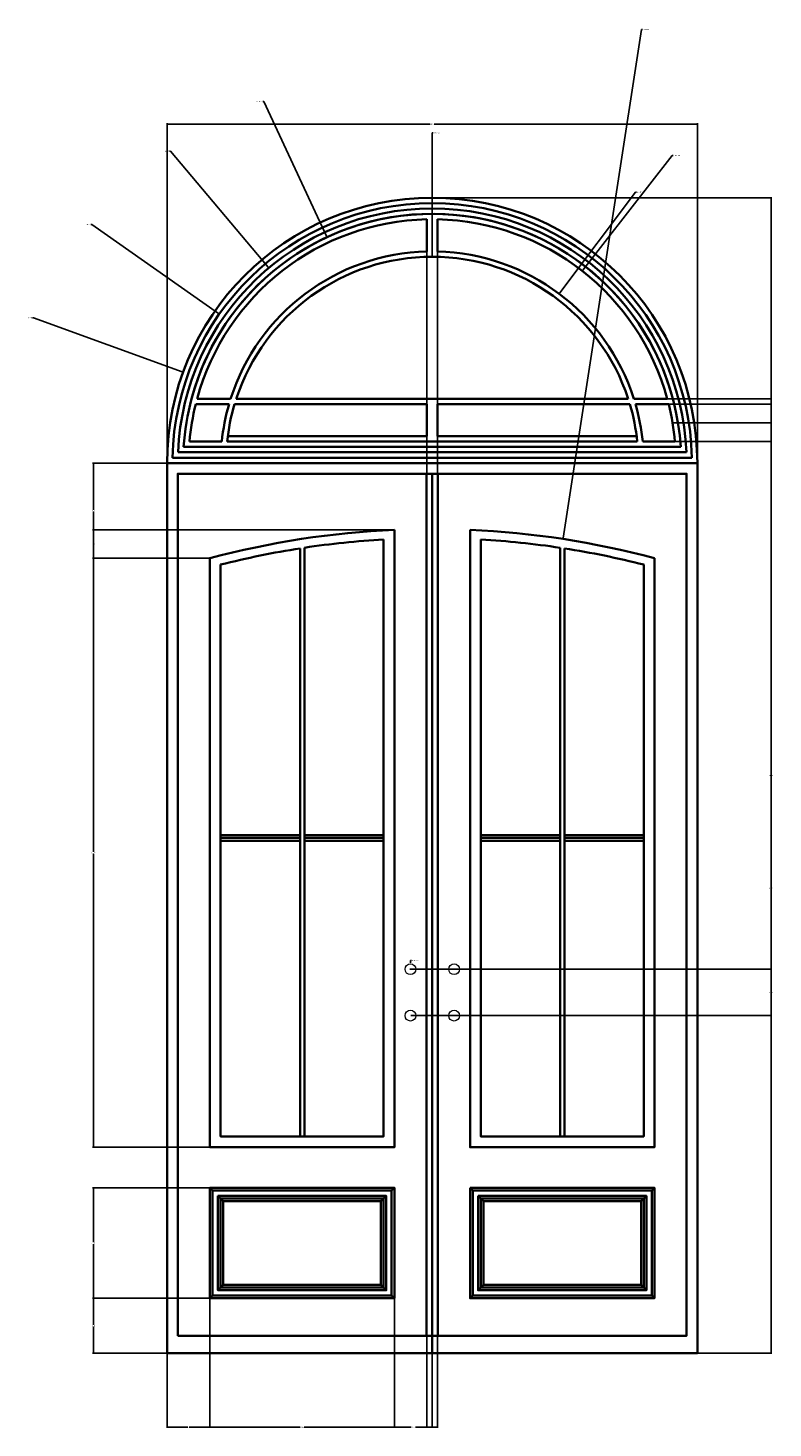
# Model space of a CAD drawing. Units: inches. Extents: x 1318 to 1980, y 617 to 1423.
# Tile 3 of 7: x 1332 to 1471, y 944 to 1205. Entities that reach past the tile are written whole.
import ezdxf

# ---------------------------------------------------------------- set-up
doc = ezdxf.new("R2010")
doc.units = ezdxf.units.IN
doc.header["$MEASUREMENT"] = 0
for name, color, linetype, lineweight in [('A-ANNO-DIMS', 2, 'Continuous', 18), ('A-DOOR', 4, 'Continuous', 35), ('A-DOOR-HDWR', 3, 'Continuous', 18)]:
    doc.layers.add(name, color=color, linetype=linetype, lineweight=lineweight)
doc.styles.get("Standard").update_dxf_attribs({"font": 'arial.ttf'})
doc.dimstyles.get("Standard").update_dxf_attribs({"dimtxt": 0.18, "dimasz": 0.18, "dimexe": 0.18, "dimexo": 0.0625, "dimgap": 0.09, "dimtad": 0, "dimtih": 1, "dimtoh": 1, "dimdec": 0, "dimzin": 0, "dimdsep": 46, "dimlunit": 3, "dimtxsty": 'Standard', "dimcen": 0.09, "dimadec": 0, "dimazin": 0, "dimtfac": 1, "dimtdec": 0, "dimtofl": 0, "dimtmove": 0, "dimatfit": 3, "dimfxl": 1, "dimtolj": 1, "dimtzin": 0, "dimarcsym": 0})

# ---------------------------------------------------------------- blocks, each defined once
blk = doc.blocks.new('DOOR-KNOB-SET')
for centre in [(1.01, 9.67), (9.16, 9.67), (1.01, 1.01), (9.16, 1.01)]:
    blk.add_circle(centre, 1.01)
blk = doc.blocks.new('*D32')
at = {"layer": 'A-ANNO-DIMS', "color": 0, "lineweight": -2, "transparency": 16777216}
for p, q in [((1403.05, 1020.69), (1470.47, 1020.69)), ((1470.29, 1020.51), (1470.29, 989.38)), ((1470.29, 957.88), (1470.29, 989.01)), ((1407.11, 957.7), (1470.47, 957.7))]:
    blk.add_line(p, q, dxfattribs=at)
at = {"layer": 'A-ANNO-DIMS', "color": 0, "transparency": 16777216}
for points in [[(1470.26, 1020.51), (1470.32, 1020.51), (1470.29, 1020.69)], [(1470.26, 957.88), (1470.32, 957.88), (1470.29, 957.7)]]:
    blk.add_solid(points, dxfattribs=at)
at = {"layer": 'Defpoints', "color": 0, "transparency": 16777216}
for p in [(1402.99, 1020.69), (1470.29, 1020.69), (1407.05, 957.7)]:
    blk.add_point(p, dxfattribs=at)
at = {"layer": 'A-ANNO-DIMS', "color": 0, "transparency": 16777216, "insert": (1470.29, 989.2), "char_height": 0.18, "attachment_point": 5}
blk.add_mtext('\\A1;63', dxfattribs=at)
blk = doc.blocks.new('*D33')
at = {"layer": 'A-ANNO-DIMS', "color": 0, "lineweight": -2, "transparency": 16777216}
for p, q in [((1403.05, 1029.36), (1470.47, 1029.36)), ((1470.29, 1029.18), (1470.29, 1025.21)), ((1470.29, 1020.87), (1470.29, 1024.84)), ((1403.05, 1020.69), (1470.47, 1020.69))]:
    blk.add_line(p, q, dxfattribs=at)
at = {"layer": 'A-ANNO-DIMS', "color": 0, "transparency": 16777216}
for points in [[(1470.26, 1029.18), (1470.32, 1029.18), (1470.29, 1029.36)], [(1470.26, 1020.87), (1470.32, 1020.87), (1470.29, 1020.69)]]:
    blk.add_solid(points, dxfattribs=at)
at = {"layer": 'Defpoints', "color": 0, "transparency": 16777216}
for p in [(1402.99, 1029.36), (1470.29, 1029.36), (1402.99, 1020.69)]:
    blk.add_point(p, dxfattribs=at)
at = {"layer": 'A-ANNO-DIMS', "color": 0, "transparency": 16777216, "insert": (1470.29, 1025.03), "char_height": 0.18, "attachment_point": 5}
blk.add_mtext('\\A1;8.663', dxfattribs=at)
blk = doc.blocks.new('*D34')
at = {"layer": 'A-ANNO-DIMS', "color": 0, "lineweight": -2, "transparency": 16777216}
for p, q in [((1357.56, 1123.84), (1357.56, 1187.2)), ((1357.74, 1187.02), (1406.65, 1187.02)), ((1456.36, 1187.02), (1407.44, 1187.02)), ((1456.54, 1123.84), (1456.54, 1187.2))]:
    blk.add_line(p, q, dxfattribs=at)
at = {"layer": 'A-ANNO-DIMS', "color": 0, "transparency": 16777216}
for points in [[(1357.74, 1187.05), (1357.74, 1186.99), (1357.56, 1187.02)], [(1456.36, 1187.05), (1456.36, 1186.99), (1456.54, 1187.02)]]:
    blk.add_solid(points, dxfattribs=at)
at = {"layer": 'Defpoints', "color": 0, "transparency": 16777216}
for p in [(1456.54, 1187.02), (1357.56, 1123.78), (1456.54, 1123.78)]:
    blk.add_point(p, dxfattribs=at)
at = {"layer": 'A-ANNO-DIMS', "color": 0, "transparency": 16777216, "insert": (1407.05, 1187.02), "char_height": 0.18, "attachment_point": 5}
blk.add_mtext('\\A1;98.98', dxfattribs=at)
blk = doc.blocks.new('*D35')
at = {"layer": 'A-ANNO-DIMS', "color": 0, "lineweight": -2, "transparency": 16777216}
for p, q in [((1451.97, 1131.3), (1470.47, 1131.3)), ((1470.29, 1131.12), (1470.29, 1044.68)), ((1470.29, 957.88), (1470.29, 1044.32)), ((1456.6, 957.7), (1470.47, 957.7))]:
    blk.add_line(p, q, dxfattribs=at)
at = {"layer": 'A-ANNO-DIMS', "color": 0, "transparency": 16777216}
for points in [[(1470.26, 1131.12), (1470.32, 1131.12), (1470.29, 1131.3)], [(1470.26, 957.88), (1470.32, 957.88), (1470.29, 957.7)]]:
    blk.add_solid(points, dxfattribs=at)
at = {"layer": 'Defpoints', "color": 0, "transparency": 16777216}
for p in [(1451.91, 1131.3), (1470.29, 1131.3), (1456.54, 957.7)]:
    blk.add_point(p, dxfattribs=at)
at = {"layer": 'A-ANNO-DIMS', "color": 0, "transparency": 16777216, "insert": (1470.29, 1044.5), "char_height": 0.18, "attachment_point": 5}
blk.add_mtext('\\A1;173.6', dxfattribs=at)
blk = doc.blocks.new('*D36')
at = {"layer": 'A-ANNO-DIMS', "color": 0, "lineweight": -2, "transparency": 16777216}
for p, q in [((1407.11, 1173.27), (1470.47, 1173.27)), ((1470.29, 1173.09), (1470.29, 1065.67)), ((1470.29, 957.88), (1470.29, 1065.3)), ((1357.62, 957.7), (1470.47, 957.7))]:
    blk.add_line(p, q, dxfattribs=at)
at = {"layer": 'A-ANNO-DIMS', "color": 0, "transparency": 16777216}
for points in [[(1470.26, 1173.09), (1470.32, 1173.09), (1470.29, 1173.27)], [(1470.26, 957.88), (1470.32, 957.88), (1470.29, 957.7)]]:
    blk.add_solid(points, dxfattribs=at)
at = {"layer": 'Defpoints', "color": 0, "transparency": 16777216}
for p in [(1407.05, 1173.27), (1470.29, 1173.27), (1357.56, 957.7)]:
    blk.add_point(p, dxfattribs=at)
at = {"layer": 'A-ANNO-DIMS', "color": 0, "transparency": 16777216, "insert": (1470.29, 1065.48), "char_height": 0.18, "attachment_point": 5}
blk.add_mtext('\\A1;215.57', dxfattribs=at)
blk = doc.blocks.new('*D37')
at = {"layer": 'A-ANNO-DIMS', "color": 0, "lineweight": -2, "transparency": 16777216}
for p, q in [((1451.249026, 1134.780871), (1470.466544, 1134.780871)), ((1470.286544, 1134.600871), (1470.286544, 1131.460871)), ((1470.286544, 1127.960871), (1470.286544, 1131.100871)), ((1452.422837, 1127.780871), (1470.466544, 1127.780871))]:
    blk.add_line(p, q, dxfattribs=at)
at = {"layer": 'A-ANNO-DIMS', "color": 0, "transparency": 16777216}
for points in [[(1470.256544, 1134.600871), (1470.316544, 1134.600871), (1470.286544, 1134.780871)], [(1470.256544, 1127.960871), (1470.316544, 1127.960871), (1470.286544, 1127.780871)]]:
    blk.add_solid(points, dxfattribs=at)
at = {"layer": 'Defpoints', "color": 0, "transparency": 16777216}
for p in [(1451.186526, 1134.780871), (1470.286544, 1134.780871), (1452.360337, 1127.780871)]:
    blk.add_point(p, dxfattribs=at)
at = {"layer": 'A-ANNO-DIMS', "color": 0, "transparency": 16777216, "insert": (1470.286544, 1131.280871), "char_height": 0.18, "attachment_point": 5}
blk.add_mtext('\\A1;7', dxfattribs=at)
blk = doc.blocks.new('*D38')
at = {"layer": 'A-ANNO-DIMS', "color": 0, "lineweight": -2, "transparency": 16777216}
for p, q in [((1450.99, 1135.78), (1470.47, 1135.78)), ((1451.25, 1134.78), (1470.47, 1134.78)), ((1470.29, 1135.6), (1470.29, 1135.46)), ((1470.29, 1134.96), (1470.29, 1135.1))]:
    blk.add_line(p, q, dxfattribs=at)
at = {"layer": 'A-ANNO-DIMS', "color": 0, "transparency": 16777216}
for points in [[(1470.26, 1135.6), (1470.32, 1135.6), (1470.29, 1135.78)], [(1470.26, 1134.96), (1470.32, 1134.96), (1470.29, 1134.78)]]:
    blk.add_solid(points, dxfattribs=at)
at = {"layer": 'Defpoints', "color": 0, "transparency": 16777216}
for p in [(1450.93, 1135.78), (1451.19, 1134.78), (1470.29, 1135.78)]:
    blk.add_point(p, dxfattribs=at)
at = {"layer": 'A-ANNO-DIMS', "color": 0, "transparency": 16777216, "insert": (1470.29, 1135.28), "char_height": 0.18, "attachment_point": 5}
blk.add_mtext('\\A1;1', dxfattribs=at)
blk = doc.blocks.new('*D39')
at = {"layer": 'A-ANNO-DIMS', "color": 0, "lineweight": -2, "transparency": 16777216}
for p, q in [((1406.05, 1163.19), (1406.05, 943.77)), ((1408.05, 1163.19), (1408.05, 943.77)), ((1406.23, 943.95), (1406.9, 943.95)), ((1407.87, 943.95), (1407.2, 943.95))]:
    blk.add_line(p, q, dxfattribs=at)
at = {"layer": 'A-ANNO-DIMS', "color": 0, "transparency": 16777216}
for points in [[(1406.23, 943.98), (1406.23, 943.92), (1406.05, 943.95)], [(1407.87, 943.98), (1407.87, 943.92), (1408.05, 943.95)]]:
    blk.add_solid(points, dxfattribs=at)
at = {"layer": 'Defpoints', "color": 0, "transparency": 16777216}
for p in [(1406.05, 1163.26), (1408.05, 1163.26), (1408.05, 943.95)]:
    blk.add_point(p, dxfattribs=at)
at = {"layer": 'A-ANNO-DIMS', "color": 0, "transparency": 16777216, "insert": (1407.05, 943.95), "char_height": 0.18, "attachment_point": 5}
blk.add_mtext('\\A1;2', dxfattribs=at)
blk = doc.blocks.new('*D40')
at = {"layer": 'A-ANNO-DIMS', "color": 0, "lineweight": -2, "transparency": 16777216}
for p, q in [((1399.92, 1111.33), (1343.63, 1111.33)), ((1343.81, 1111.15), (1343.81, 1108.86)), ((1343.81, 1106.2), (1343.81, 1108.49)), ((1365.5, 1106.02), (1343.63, 1106.02))]:
    blk.add_line(p, q, dxfattribs=at)
at = {"layer": 'A-ANNO-DIMS', "color": 0, "transparency": 16777216}
for points in [[(1343.78, 1111.15), (1343.84, 1111.15), (1343.81, 1111.33)], [(1343.78, 1106.2), (1343.84, 1106.2), (1343.81, 1106.02)]]:
    blk.add_solid(points, dxfattribs=at)
at = {"layer": 'Defpoints', "color": 0, "transparency": 16777216}
for p in [(1343.81, 1111.33), (1399.98, 1111.33), (1365.56, 1106.02)]:
    blk.add_point(p, dxfattribs=at)
at = {"layer": 'A-ANNO-DIMS', "color": 0, "transparency": 16777216, "insert": (1343.81, 1108.68), "char_height": 0.18, "attachment_point": 5}
blk.add_mtext('\\A1;5.306', dxfattribs=at)
blk = doc.blocks.new('*D41')
at = {"layer": 'A-ANNO-DIMS', "color": 0, "lineweight": -2, "transparency": 16777216}
for p, q in [((1365.56, 967.92), (1365.56, 943.77)), ((1357.56, 957.63), (1357.56, 943.77)), ((1357.74, 943.95), (1361.41, 943.95)), ((1365.38, 943.95), (1361.71, 943.95))]:
    blk.add_line(p, q, dxfattribs=at)
at = {"layer": 'A-ANNO-DIMS', "color": 0, "transparency": 16777216}
for points in [[(1357.74, 943.98), (1357.74, 943.92), (1357.56, 943.95)], [(1365.38, 943.98), (1365.38, 943.92), (1365.56, 943.95)]]:
    blk.add_solid(points, dxfattribs=at)
at = {"layer": 'Defpoints', "color": 0, "transparency": 16777216}
for p in [(1365.56, 967.98), (1357.56, 957.7), (1365.56, 943.95)]:
    blk.add_point(p, dxfattribs=at)
at = {"layer": 'A-ANNO-DIMS', "color": 0, "transparency": 16777216, "insert": (1361.56, 943.95), "char_height": 0.18, "attachment_point": 5}
blk.add_mtext('\\A1;8', dxfattribs=at)
blk = doc.blocks.new('*D42')
at = {"layer": 'A-ANNO-DIMS', "color": 0, "lineweight": -2, "transparency": 16777216}
for p, q in [((1365.56, 967.92), (1365.56, 943.77)), ((1399.98, 967.92), (1399.98, 943.77)), ((1365.74, 943.95), (1382.38, 943.95)), ((1399.8, 943.95), (1383.16, 943.95))]:
    blk.add_line(p, q, dxfattribs=at)
at = {"layer": 'A-ANNO-DIMS', "color": 0, "transparency": 16777216}
for points in [[(1365.74, 943.98), (1365.74, 943.92), (1365.56, 943.95)], [(1399.8, 943.98), (1399.8, 943.92), (1399.98, 943.95)]]:
    blk.add_solid(points, dxfattribs=at)
at = {"layer": 'Defpoints', "color": 0, "transparency": 16777216}
for p in [(1365.56, 967.98), (1399.98, 967.98), (1399.98, 943.95)]:
    blk.add_point(p, dxfattribs=at)
at = {"layer": 'A-ANNO-DIMS', "color": 0, "transparency": 16777216, "insert": (1382.77, 943.95), "char_height": 0.18, "attachment_point": 5}
blk.add_mtext('\\A1;34.42', dxfattribs=at)
blk = doc.blocks.new('*D43')
at = {"layer": 'A-ANNO-DIMS', "color": 0, "lineweight": -2, "transparency": 16777216}
for p, q in [((1399.98, 967.92), (1399.98, 943.77)), ((1407.05, 957.63), (1407.05, 943.77)), ((1400.16, 943.95), (1403.12, 943.95)), ((1406.87, 943.95), (1403.91, 943.95))]:
    blk.add_line(p, q, dxfattribs=at)
at = {"layer": 'A-ANNO-DIMS', "color": 0, "transparency": 16777216}
for points in [[(1400.16, 943.98), (1400.16, 943.92), (1399.98, 943.95)], [(1406.87, 943.98), (1406.87, 943.92), (1407.05, 943.95)]]:
    blk.add_solid(points, dxfattribs=at)
at = {"layer": 'Defpoints', "color": 0, "transparency": 16777216}
for p in [(1399.98, 967.98), (1407.05, 957.7), (1407.05, 943.95)]:
    blk.add_point(p, dxfattribs=at)
at = {"layer": 'A-ANNO-DIMS', "color": 0, "transparency": 16777216, "insert": (1403.51, 943.95), "char_height": 0.18, "attachment_point": 5}
blk.add_mtext('\\A1;7.068', dxfattribs=at)
blk = doc.blocks.new('*D44')
at = {"layer": 'A-ANNO-DIMS', "color": 0, "lineweight": -2, "transparency": 16777216}
for p, q in [((1365.5, 967.98), (1343.63, 967.98)), ((1343.81, 967.8), (1343.81, 963.02)), ((1343.81, 957.88), (1343.81, 962.66)), ((1357.5, 957.7), (1343.63, 957.7))]:
    blk.add_line(p, q, dxfattribs=at)
at = {"layer": 'A-ANNO-DIMS', "color": 0, "transparency": 16777216}
for points in [[(1343.78, 967.8), (1343.84, 967.8), (1343.81, 967.98)], [(1343.78, 957.88), (1343.84, 957.88), (1343.81, 957.7)]]:
    blk.add_solid(points, dxfattribs=at)
at = {"layer": 'Defpoints', "color": 0, "transparency": 16777216}
for p in [(1343.81, 967.98), (1365.56, 967.98), (1357.56, 957.7)]:
    blk.add_point(p, dxfattribs=at)
at = {"layer": 'A-ANNO-DIMS', "color": 0, "transparency": 16777216, "insert": (1343.81, 962.84), "char_height": 0.18, "attachment_point": 5}
blk.add_mtext('\\A1;10.28', dxfattribs=at)
blk = doc.blocks.new('*D45')
at = {"layer": 'A-ANNO-DIMS', "color": 0, "lineweight": -2, "transparency": 16777216}
for p, q in [((1365.5, 988.57), (1343.63, 988.57)), ((1343.81, 988.39), (1343.81, 978.46)), ((1343.81, 968.16), (1343.81, 978.09)), ((1365.5, 967.98), (1343.63, 967.98))]:
    blk.add_line(p, q, dxfattribs=at)
at = {"layer": 'A-ANNO-DIMS', "color": 0, "transparency": 16777216}
for points in [[(1343.78, 988.39), (1343.84, 988.39), (1343.81, 988.57)], [(1343.78, 968.16), (1343.84, 968.16), (1343.81, 967.98)]]:
    blk.add_solid(points, dxfattribs=at)
at = {"layer": 'Defpoints', "color": 0, "transparency": 16777216}
for p in [(1343.81, 988.57), (1365.56, 988.57), (1365.56, 967.98)]:
    blk.add_point(p, dxfattribs=at)
at = {"layer": 'A-ANNO-DIMS', "color": 0, "transparency": 16777216, "insert": (1343.81, 978.28), "char_height": 0.18, "attachment_point": 5}
blk.add_mtext('\\A1;20.596', dxfattribs=at)
blk = doc.blocks.new('*D46')
at = {"layer": 'A-ANNO-DIMS', "color": 0, "lineweight": -2, "transparency": 16777216}
for p, q in [((1365.5, 1106.02), (1343.63, 1106.02)), ((1343.81, 1105.84), (1343.81, 1051.27)), ((1343.81, 996.34), (1343.81, 1050.91)), ((1365.5, 996.16), (1343.63, 996.16))]:
    blk.add_line(p, q, dxfattribs=at)
at = {"layer": 'A-ANNO-DIMS', "color": 0, "transparency": 16777216}
for points in [[(1343.78, 1105.84), (1343.84, 1105.84), (1343.81, 1106.02)], [(1343.78, 996.34), (1343.84, 996.34), (1343.81, 996.16)]]:
    blk.add_solid(points, dxfattribs=at)
at = {"layer": 'Defpoints', "color": 0, "transparency": 16777216}
for p in [(1343.81, 1106.02), (1365.56, 1106.02), (1365.56, 996.16)]:
    blk.add_point(p, dxfattribs=at)
at = {"layer": 'A-ANNO-DIMS', "color": 0, "transparency": 16777216, "insert": (1343.81, 1051.09), "char_height": 0.18, "attachment_point": 5}
blk.add_mtext('\\A1;109.87', dxfattribs=at)
blk = doc.blocks.new('*D47')
at = {"layer": 'A-ANNO-DIMS', "color": 0, "lineweight": -2, "transparency": 16777216}
for p, q in [((1357.5, 1123.78), (1343.63, 1123.78)), ((1343.81, 1123.6), (1343.81, 1115.08)), ((1343.81, 1106.2), (1343.81, 1114.72)), ((1365.5, 1106.02), (1343.63, 1106.02))]:
    blk.add_line(p, q, dxfattribs=at)
at = {"layer": 'A-ANNO-DIMS', "color": 0, "transparency": 16777216}
for points in [[(1343.78, 1123.6), (1343.84, 1123.6), (1343.81, 1123.78)], [(1343.78, 1106.2), (1343.84, 1106.2), (1343.81, 1106.02)]]:
    blk.add_solid(points, dxfattribs=at)
at = {"layer": 'Defpoints', "color": 0, "transparency": 16777216}
for p in [(1343.81, 1123.78), (1357.56, 1123.78), (1365.56, 1106.02)]:
    blk.add_point(p, dxfattribs=at)
at = {"layer": 'A-ANNO-DIMS', "color": 0, "transparency": 16777216, "insert": (1343.81, 1114.9), "char_height": 0.18, "attachment_point": 5}
blk.add_mtext('\\A1;17.76', dxfattribs=at)
blk = doc.blocks.new('*D105')
at = {"layer": 'A-ANNO-DIMS', "color": 0, "lineweight": -2, "transparency": 16777216}
for p, q in [((1332.46, 1150.87), (1332.64, 1150.87)), ((1332.64, 1150.87), (1360.37, 1140.77)), ((1406.96, 1123.78), (1407.14, 1123.78)), ((1407.05, 1123.69), (1407.05, 1123.87))]:
    blk.add_line(p, q, dxfattribs=at)
at = {"layer": 'A-ANNO-DIMS', "color": 0, "transparency": 16777216}
blk.add_solid([(1360.38, 1140.8), (1360.36, 1140.74), (1360.54, 1140.71)], dxfattribs=at)
at = {"layer": 'Defpoints', "color": 0, "transparency": 16777216}
for p in [(1360.54, 1140.71), (1407.05, 1123.78)]:
    blk.add_point(p, dxfattribs=at)
at = {"layer": 'A-ANNO-DIMS', "color": 0, "transparency": 16777216, "insert": (1331.98, 1150.87), "char_height": 0.18, "attachment_point": 5}
blk.add_mtext('\\A1;R49.49', dxfattribs=at)
blk = doc.blocks.new('*D106')
at = {"layer": 'A-ANNO-DIMS', "color": 0, "lineweight": -2, "transparency": 16777216}
for p, q in [((1343.31, 1168.28), (1343.49, 1168.28)), ((1343.49, 1168.28), (1367.18, 1151.7)), ((1406.96, 1123.78), (1407.14, 1123.78)), ((1407.05, 1123.69), (1407.05, 1123.87))]:
    blk.add_line(p, q, dxfattribs=at)
at = {"layer": 'A-ANNO-DIMS', "color": 0, "transparency": 16777216}
blk.add_solid([(1367.2, 1151.72), (1367.16, 1151.67), (1367.33, 1151.59)], dxfattribs=at)
at = {"layer": 'Defpoints', "color": 0, "transparency": 16777216}
for p in [(1367.33, 1151.59), (1407.05, 1123.78)]:
    blk.add_point(p, dxfattribs=at)
at = {"layer": 'A-ANNO-DIMS', "color": 0, "transparency": 16777216, "insert": (1342.83, 1168.28), "char_height": 0.18, "attachment_point": 5}
blk.add_mtext('\\A1;R48.49', dxfattribs=at)
blk = doc.blocks.new('*D107')
at = {"layer": 'A-ANNO-DIMS', "color": 0, "lineweight": -2, "transparency": 16777216}
for p, q in [((1358.03, 1181.99), (1358.21, 1181.99)), ((1358.21, 1181.99), (1376.41, 1160.3)), ((1406.96, 1123.78), (1407.14, 1123.78)), ((1407.05, 1123.69), (1407.05, 1123.87))]:
    blk.add_line(p, q, dxfattribs=at)
at = {"layer": 'A-ANNO-DIMS', "color": 0, "transparency": 16777216}
blk.add_solid([(1376.43, 1160.32), (1376.38, 1160.28), (1376.52, 1160.16)], dxfattribs=at)
at = {"layer": 'Defpoints', "color": 0, "transparency": 16777216}
for p in [(1376.52, 1160.16), (1407.05, 1123.78)]:
    blk.add_point(p, dxfattribs=at)
at = {"layer": 'A-ANNO-DIMS', "color": 0, "transparency": 16777216, "insert": (1357.55, 1181.99), "char_height": 0.18, "attachment_point": 5}
blk.add_mtext('\\A1;R47.49', dxfattribs=at)
blk = doc.blocks.new('*D108')
at = {"layer": 'A-ANNO-DIMS', "color": 0, "lineweight": -2, "transparency": 16777216}
for p, q in [((1375.44, 1191.2), (1375.62, 1191.2)), ((1375.62, 1191.2), (1387.33, 1166.08)), ((1406.96, 1123.78), (1407.14, 1123.78)), ((1407.05, 1123.69), (1407.05, 1123.87))]:
    blk.add_line(p, q, dxfattribs=at)
at = {"layer": 'A-ANNO-DIMS', "color": 0, "transparency": 16777216}
blk.add_solid([(1387.35, 1166.09), (1387.3, 1166.07), (1387.4, 1165.92)], dxfattribs=at)
at = {"layer": 'Defpoints', "color": 0, "transparency": 16777216}
for p in [(1387.4, 1165.92), (1407.05, 1123.78)]:
    blk.add_point(p, dxfattribs=at)
at = {"layer": 'A-ANNO-DIMS', "color": 0, "transparency": 16777216, "insert": (1374.76, 1191.2), "char_height": 0.18, "attachment_point": 5}
blk.add_mtext('\\A1;3X R46.49', dxfattribs=at)
blk = doc.blocks.new('*D109')
at = {"layer": 'A-ANNO-DIMS', "color": 0, "lineweight": -2, "transparency": 16777216}
for p, q in [((1451.84, 1181.15), (1435.15, 1159.78)), ((1452.02, 1181.15), (1451.84, 1181.15)), ((1406.96, 1123.78), (1407.14, 1123.78)), ((1407.05, 1123.69), (1407.05, 1123.87))]:
    blk.add_line(p, q, dxfattribs=at)
at = {"layer": 'A-ANNO-DIMS', "color": 0, "transparency": 16777216}
blk.add_solid([(1435.13, 1159.8), (1435.18, 1159.76), (1435.04, 1159.64)], dxfattribs=at)
at = {"layer": 'Defpoints', "color": 0, "transparency": 16777216}
for p in [(1435.04, 1159.64), (1407.05, 1123.78)]:
    blk.add_point(p, dxfattribs=at)
at = {"layer": 'A-ANNO-DIMS', "color": 0, "transparency": 16777216, "insert": (1452.7, 1181.15), "char_height": 0.18, "attachment_point": 5}
blk.add_mtext('\\A1;4X R45.49', dxfattribs=at)
blk = doc.blocks.new('*D110')
at = {"layer": 'A-ANNO-DIMS', "color": 0, "lineweight": -2, "transparency": 16777216}
for p, q in [((1444.97, 1174.32), (1430.85, 1155.51)), ((1445.15, 1174.32), (1444.97, 1174.32)), ((1406.96, 1123.78), (1407.14, 1123.78)), ((1407.05, 1123.69), (1407.05, 1123.87))]:
    blk.add_line(p, q, dxfattribs=at)
at = {"layer": 'A-ANNO-DIMS', "color": 0, "transparency": 16777216}
blk.add_solid([(1430.83, 1155.53), (1430.88, 1155.49), (1430.75, 1155.37)], dxfattribs=at)
at = {"layer": 'Defpoints', "color": 0, "transparency": 16777216}
for p in [(1430.75, 1155.37), (1407.05, 1123.78)]:
    blk.add_point(p, dxfattribs=at)
at = {"layer": 'A-ANNO-DIMS', "color": 0, "transparency": 16777216, "insert": (1445.82, 1174.32), "char_height": 0.18, "attachment_point": 5}
blk.add_mtext('\\A1;4X R39.49', dxfattribs=at)
blk = doc.blocks.new('*D111')
at = {"layer": 'A-ANNO-DIMS', "color": 0, "lineweight": -2, "transparency": 16777216}
for p, q in [((1407.23, 1185.36), (1407.05, 1185.36)), ((1407.05, 1185.36), (1407.05, 1162.45)), ((1406.96, 1123.78), (1407.14, 1123.78)), ((1407.05, 1123.69), (1407.05, 1123.87))]:
    blk.add_line(p, q, dxfattribs=at)
at = {"layer": 'A-ANNO-DIMS', "color": 0, "transparency": 16777216}
blk.add_solid([(1407.02, 1162.45), (1407.08, 1162.45), (1407.05, 1162.27)], dxfattribs=at)
at = {"layer": 'Defpoints', "color": 0, "transparency": 16777216}
for p in [(1407.05, 1162.27), (1407.05, 1123.78)]:
    blk.add_point(p, dxfattribs=at)
at = {"layer": 'A-ANNO-DIMS', "color": 0, "transparency": 16777216, "insert": (1407.9, 1185.36), "char_height": 0.18, "attachment_point": 5}
blk.add_mtext('\\A1;3X R38.49', dxfattribs=at)
blk = doc.blocks.new('*D112')
at = {"layer": 'A-ANNO-DIMS', "color": 0, "lineweight": -2, "transparency": 16777216}
for p, q in [((1446.12, 1204.67), (1431.5, 1109.79)), ((1446.3, 1204.67), (1446.12, 1204.67)), ((1406.96, 951.18), (1407.14, 951.18)), ((1407.05, 951.09), (1407.05, 951.27))]:
    blk.add_line(p, q, dxfattribs=at)
at = {"layer": 'A-ANNO-DIMS', "color": 0, "transparency": 16777216}
blk.add_solid([(1431.47, 1109.8), (1431.53, 1109.79), (1431.47, 1109.61)], dxfattribs=at)
at = {"layer": 'Defpoints', "color": 0, "transparency": 16777216}
for p in [(1431.47, 1109.61), (1407.05, 951.18)]:
    blk.add_point(p, dxfattribs=at)
at = {"layer": 'A-ANNO-DIMS', "color": 0, "transparency": 16777216, "insert": (1446.98, 1204.67), "char_height": 0.18, "attachment_point": 5}
blk.add_mtext('\\A1;6X R160.3', dxfattribs=at)
blk = doc.blocks.new('*D113')
at = {"layer": 'A-ANNO-DIMS', "color": 0, "lineweight": -2, "transparency": 16777216}
for p, q in [((1402.9, 1029.36), (1403.08, 1029.36)), ((1402.99, 1029.27), (1402.99, 1029.45)), ((1403.01, 1030.97), (1403, 1030.55)), ((1403.19, 1030.97), (1403.01, 1030.97))]:
    blk.add_line(p, q, dxfattribs=at)
at = {"layer": 'A-ANNO-DIMS', "color": 0, "transparency": 16777216}
blk.add_solid([(1402.97, 1030.55), (1403.03, 1030.54), (1403, 1030.37)], dxfattribs=at)
at = {"layer": 'Defpoints', "color": 0, "transparency": 16777216}
for p in [(1403, 1030.37), (1402.97, 1028.35)]:
    blk.add_point(p, dxfattribs=at)
at = {"layer": 'A-ANNO-DIMS', "color": 0, "transparency": 16777216, "insert": (1403.87, 1030.97), "char_height": 0.18, "attachment_point": 5}
blk.add_mtext('\\A1;4X ∅2.017', dxfattribs=at)

msp = doc.modelspace()

# ---------------------------------------------------------------- linework, layer by layer
at = {"layer": 'A-DOOR'}
for p, q in [((1406.0473, 1163.2574), (1406.0473, 1169.2591)), ((1408.0473, 1163.2574), (1408.0473, 1169.2591)), ((1362.9081, 1134.7809), (1369.1211, 1134.7809)), ((1363.1694, 1135.7809), (1369.4255, 1135.7809)), ((1370.1634, 1134.7809), (1406.0473, 1134.7809)), ((1370.4765, 1135.7809), (1443.6181, 1135.7809)), ((1406.0473, 1128.7809), (1406.0473, 1134.7809)), ((1408.0473, 1128.7809), (1408.0473, 1134.7809)), ((1408.0473, 1134.7809), (1443.9312, 1134.7809)), ((1444.6691, 1135.7809), (1450.9252, 1135.7809)), ((1444.9735, 1134.7809), (1451.1865, 1134.7809)), ((1368.8842, 1128.7809), (1406.0473, 1128.7809)), ((1408.0473, 1128.7809), (1445.2104, 1128.7809)), ((1452.2609, 1128.7809), (1452.3603, 1128.7809)), ((1359.6002, 1125.7809), (1454.4944, 1125.7809)), ((1360.655, 1126.7809), (1453.4396, 1126.7809)), ((1361.7343, 1127.7809), (1367.7612, 1127.7809)), ((1368.7665, 1127.7809), (1445.3281, 1127.7809)), ((1446.3334, 1127.7809), (1452.3603, 1127.7809)), ((1357.5581, 1124.7809), (1357.5682, 1124.7809)), ((1357.5581, 1123.7809), (1456.5365, 1123.7809)), ((1358.5684, 1124.7809), (1455.5262, 1124.7809)), ((1456.5264, 1124.7809), (1456.5365, 1124.7809)), ((1405.9793, 960.9905), (1405.9793, 1121.7809)), ((1407.0473, 960.9905), (1407.0473, 1121.7809)), ((1408.1153, 960.9905), (1408.1153, 1121.7809)), ((1382.3748, 1107.8593), (1382.3748, 998.1571)), ((1383.1983, 1107.9854), (1383.1983, 998.1571)), ((1430.932, 1107.98), (1430.932, 998.1571)), ((1431.7555, 1107.8538), (1431.7555, 998.1571)), ((1367.5581, 1054.3349), (1382.3748, 1054.3349)), ((1367.5581, 1053.8349), (1382.3748, 1053.8349)), ((1367.5581, 1053.3349), (1382.3748, 1053.3349)), ((1383.1983, 1054.3349), (1397.9793, 1054.3349)), ((1383.1983, 1053.8349), (1397.9793, 1053.8349)), ((1383.1983, 1053.3349), (1397.9793, 1053.3349)), ((1416.1153, 1054.3349), (1430.932, 1054.3349)), ((1416.1153, 1053.8349), (1430.932, 1053.8349)), ((1416.1153, 1053.3349), (1430.932, 1053.3349)), ((1431.7555, 1054.3349), (1446.5365, 1054.3349)), ((1431.7555, 1053.8349), (1446.5365, 1053.8349)), ((1431.7555, 1053.3349), (1446.5365, 1053.3349)), ((1365.5581, 988.5731), (1366.0581, 988.0731)), ((1399.4793, 988.0731), (1399.9793, 988.5731)), ((1414.1153, 988.5731), (1414.6153, 988.0731)), ((1448.0365, 988.0731), (1448.5365, 988.5731)), ((1367.0581, 987.0731), (1368.0581, 986.0731)), ((1397.4793, 986.0731), (1398.4793, 987.0731)), ((1415.6153, 987.0731), (1416.6153, 986.0731)), ((1446.0365, 986.0731), (1447.0365, 987.0731)), ((1367.0581, 969.4775), (1368.0581, 970.4775)), ((1398.4793, 969.4775), (1397.4793, 970.4775)), ((1415.6153, 969.4775), (1416.6153, 970.4775)), ((1447.0365, 969.4775), (1446.0365, 970.4775)), ((1365.5581, 967.9775), (1366.0581, 968.4775)), ((1399.9793, 967.9775), (1399.4793, 968.4775)), ((1414.1153, 967.9775), (1414.6153, 968.4775)), ((1448.5365, 967.9775), (1448.0365, 968.4775)), ((1407.0473, 960.9905), (1407.0473, 957.6972))]:
    msp.add_line(p, q, dxfattribs=at)
for points in [[(1357.5581, 1123.7809), (1456.5365, 1123.7809), (1456.5365, 957.6972), (1357.5581, 957.6972)], [(1359.5581, 960.9905), (1359.5581, 1121.7809), (1454.5365, 1121.7809), (1454.5365, 960.9905)], [(1365.5581, 988.5731), (1399.9793, 988.5731), (1399.9793, 967.9775), (1365.5581, 967.9775)], [(1366.0581, 988.0731), (1399.4793, 988.0731), (1399.4793, 968.4775), (1366.0581, 968.4775)], [(1414.1153, 988.5731), (1448.5365, 988.5731), (1448.5365, 967.9775), (1414.1153, 967.9775)], [(1414.6153, 988.0731), (1448.0365, 988.0731), (1448.0365, 968.4775), (1414.6153, 968.4775)], [(1367.0581, 987.0731), (1398.4793, 987.0731), (1398.4793, 969.4775), (1367.0581, 969.4775)], [(1367.5581, 986.5731), (1397.9793, 986.5731), (1397.9793, 969.9775), (1367.5581, 969.9775)], [(1368.0581, 986.0731), (1397.4793, 986.0731), (1397.4793, 970.4775), (1368.0581, 970.4775)], [(1415.6153, 987.0731), (1447.0365, 987.0731), (1447.0365, 969.4775), (1415.6153, 969.4775)], [(1416.1153, 986.5731), (1446.5365, 986.5731), (1446.5365, 969.9775), (1416.1153, 969.9775)], [(1416.6153, 986.0731), (1446.0365, 986.0731), (1446.0365, 970.4775), (1416.6153, 970.4775)]]:
    msp.add_lwpolyline(points, close=True, dxfattribs=at)
for points in [[(1399.9793, 1111.3286), (1399.9793, 996.1571), (1365.5581, 996.1571), (1365.5581, 1106.0223)], [(1448.5365, 1106.0223), (1448.5365, 996.1571), (1414.1153, 996.1571), (1414.1153, 1111.3286)], [(1397.9793, 1109.5127), (1397.9793, 998.1571), (1367.5581, 998.1571), (1367.5581, 1104.8294)], [(1446.5365, 1104.8294), (1446.5365, 998.1571), (1416.1153, 998.1571), (1416.1153, 1109.5127)]]:
    msp.add_lwpolyline(points, dxfattribs=at)
for centre, radius, start, end in [((1407.0473, 1123.7809), 49.4892, 0, 180), ((1407.0473, 1123.7809), 48.4892, 1.181702, 178.818298), ((1407.0473, 1123.7809), 47.4892, 2.413715, 177.586285), ((1407.0473, 1123.7809), 46.4892, 3.699929, 165.041208), ((1407.0473, 1123.7809), 46.4892, 14.958792, 165.041208), ((1407.0473, 1123.7809), 45.4892, 91.259647, 164.704418), ((1407.0473, 1123.7809), 45.4892, 15.295582, 88.740353), ((1407.0473, 1123.7809), 39.4892, 91.451077, 162.309189), ((1407.0473, 1123.7809), 38.4892, 18.166261, 161.833739), ((1407.0473, 1123.7809), 39.4892, 17.690811, 88.548923), ((1407.0473, 1123.7809), 46.4892, 165.041208, 176.300071), ((1407.0473, 1123.7809), 45.4892, 166.006286, 174.955301), ((1407.0473, 1123.7809), 39.4892, 163.825904, 174.186344), ((1407.0473, 1123.7809), 38.4892, 163.393673, 174.034756), ((1407.0473, 1123.7809), 38.4892, 5.965244, 16.606327), ((1407.0473, 1123.7809), 39.4892, 5.813656, 16.174096), ((1407.0473, 1123.7809), 45.4892, 5.044699, 13.993714), ((1407.0473, 951.1824), 160.3021, 92.527078, 105), ((1407.0473, 951.1824), 160.3021, 75, 87.472922), ((1407.0473, 949.4673), 160.3021, 98.853734, 104.261191), ((1407.0473, 949.4673), 160.3021, 93.242837, 98.555952), ((1407.0473, 949.4673), 160.3021, 81.431136, 86.757163), ((1407.0473, 949.4673), 160.3021, 75.738809, 81.133343)]:
    msp.add_arc(centre, radius, start, end, dxfattribs=at)

# ---------------------------------------------------------------- block references
at = {"layer": 'A-DOOR-HDWR'}
msp.add_blockref('DOOR-KNOB-SET', (1401.9776, 1019.6853), dxfattribs=at)

# ---------------------------------------------------------------- dimensions: what is measured, and where the dimension line sits
at = {"layer": 'A-ANNO-DIMS'}
for center, mpoint, text, override, picture, middle in [((1407.0473, 951.1824), (1431.4704, 1109.613), '6X <>', {"dimdec": 1, "dimlfac": 1, "dimrnd": 0, "dimzin": 0, "dimdsep": 46, "dimlunit": 2}, '*D112', (1446.978, 1204.6714)), ((1407.0473, 1123.7809), (1387.4022, 1165.9154), '3X <>', {"dimdec": 2, "dimlfac": 1, "dimrnd": 0, "dimzin": 0, "dimdsep": 46, "dimlunit": 2}, '*D108', (1374.7617, 1191.1961)), ((1407.0473, 1123.7809), (1407.05, 1162.2701), '3X <>', {"dimdec": 2, "dimlfac": 1, "dimrnd": 0, "dimzin": 0, "dimdsep": 46, "dimlunit": 2}, '*D111', (1407.905, 1185.3637)), ((1407.0473, 1123.7809), (1435.0418, 1159.6358), '4X <>', {"dimdec": 2, "dimlfac": 1, "dimrnd": 0, "dimzin": 0, "dimdsep": 46, "dimlunit": 2}, '*D109', (1452.6956, 1181.1488)), ((1407.0473, 1123.7809), (1430.7462, 1155.3683), '4X <>', {"dimdec": 2, "dimlfac": 1, "dimrnd": 0, "dimzin": 0, "dimdsep": 46, "dimlunit": 2}, '*D110', (1445.8225, 1174.3207))]:
    dim = msp.add_radius_dim(center=center, mpoint=mpoint, text=text, dimstyle='Standard', override=override, dxfattribs=at)
    dim.commit()
    dim.dimension.update_dxf_attribs({"geometry": picture, "text_midpoint": middle, "dimtype": 164})
for base, p1, p2, override, picture, middle in [((1456.5365, 1187.0201), (1357.5581, 1123.7809), (1456.5365, 1123.7809), {"dimdec": 2, "dimlfac": 1, "dimrnd": 0, "dimzin": 0, "dimdsep": 46, "dimlunit": 2}, '*D34', (1407.0473, 1187.0201)), ((1408.0473, 943.9472), (1406.0473, 1163.2574), (1408.0473, 1163.2574), {"dimdec": 0, "dimlfac": 1, "dimrnd": 0, "dimzin": 0, "dimdsep": 46, "dimlunit": 2}, '*D39', (1407.0473, 943.9472)), ((1365.5581, 943.9472), (1357.5581, 957.6972), (1365.5581, 967.9775), {"dimdec": 0, "dimlfac": 1, "dimrnd": 0, "dimzin": 0, "dimdsep": 46, "dimlunit": 2}, '*D41', (1361.5581, 943.9472)), ((1399.9793, 943.9472), (1365.5581, 967.9775), (1399.9793, 967.9775), {"dimdec": 2, "dimlfac": 1, "dimrnd": 0, "dimzin": 0, "dimdsep": 46, "dimlunit": 2}, '*D42', (1382.7687, 943.9472)), ((1407.0473, 943.9472), (1399.9793, 967.9775), (1407.0473, 957.6972), {"dimdec": 3, "dimlfac": 1, "dimrnd": 0, "dimzin": 0, "dimdsep": 46, "dimlunit": 2}, '*D43', (1403.5133, 943.9472))]:
    dim = msp.add_linear_dim(base=base, p1=p1, p2=p2, dimstyle='Standard', override=override, dxfattribs=at)
    dim.commit()
    dim.dimension.update_dxf_attribs({"geometry": picture, "text_midpoint": middle})
for mpoint, picture, middle in [((1376.5209, 1160.159), '*D107', (1357.545, 1181.9858)), ((1367.3267, 1151.5923), '*D106', (1342.8343, 1168.2792)), ((1360.5432, 1140.7088), '*D105', (1331.9808, 1150.8656))]:
    dim = msp.add_radius_dim(center=(1407.0473, 1123.7809), mpoint=mpoint, dimstyle='Standard', override={"dimdec": 2, "dimlfac": 1, "dimrnd": 0, "dimzin": 0, "dimdsep": 46, "dimlunit": 2}, dxfattribs=at)
    dim.commit()
    dim.dimension.update_dxf_attribs({"geometry": picture, "text_midpoint": middle, "dimtype": 164})
for base, p1, p2, override, picture, middle in [((1470.2865, 1173.2701), (1357.5581, 957.6972), (1407.0473, 1173.2701), {"dimdec": 2, "dimlfac": 1, "dimrnd": 0, "dimzin": 0, "dimdsep": 46, "dimlunit": 2}, '*D36', (1470.2865, 1065.4836)), ((1470.2865, 1135.7809), (1451.1865, 1134.7809), (1450.9252, 1135.7809), {"dimdec": 0, "dimlfac": 1, "dimrnd": 0, "dimzin": 0, "dimdsep": 46, "dimlunit": 2}, '*D38', (1470.2865, 1135.2809)), ((1470.2865, 1134.7809), (1452.3603, 1127.7809), (1451.1865, 1134.7809), {"dimdec": 0, "dimlfac": 1, "dimrnd": 0, "dimzin": 0, "dimdsep": 46, "dimlunit": 2}, '*D37', (1470.2865, 1131.2809)), ((1470.2865, 1131.3038), (1456.5365, 957.6972), (1451.9102, 1131.3038), {"dimdec": 1, "dimlfac": 1, "dimrnd": 0, "dimzin": 0, "dimdsep": 46, "dimlunit": 2}, '*D35', (1470.2865, 1044.5005)), ((1343.8081, 1123.7809), (1365.5581, 1106.0223), (1357.5581, 1123.7809), {"dimdec": 2, "dimlfac": 1, "dimrnd": 0, "dimzin": 0, "dimdsep": 46, "dimlunit": 2}, '*D47', (1343.8081, 1114.9016)), ((1343.8081, 1111.3286), (1365.5581, 1106.0223), (1399.9793, 1111.3286), {"dimdec": 3, "dimlfac": 1, "dimrnd": 0, "dimzin": 0, "dimdsep": 46, "dimlunit": 2}, '*D40', (1343.8081, 1108.6754)), ((1343.8081, 1106.0223), (1365.5581, 996.1571), (1365.5581, 1106.0223), {"dimdec": 2, "dimlfac": 1, "dimrnd": 0, "dimzin": 0, "dimdsep": 46, "dimlunit": 2}, '*D46', (1343.8081, 1051.0897)), ((1470.2865, 1029.3567), (1402.9866, 1020.6939), (1402.9866, 1029.3567), {"dimdec": 3, "dimlfac": 1, "dimrnd": 0, "dimzin": 0, "dimdsep": 46, "dimlunit": 2}, '*D33', (1470.2865, 1025.0253)), ((1470.2865, 1020.6939), (1407.0473, 957.6972), (1402.9866, 1020.6939), {"dimdec": 0, "dimlfac": 1, "dimrnd": 0, "dimzin": 0, "dimdsep": 46, "dimlunit": 2}, '*D32', (1470.2865, 989.1955)), ((1343.8081, 988.5731), (1365.5581, 967.9775), (1365.5581, 988.5731), {"dimdec": 3, "dimlfac": 1, "dimrnd": 0, "dimzin": 0, "dimdsep": 46, "dimlunit": 2}, '*D45', (1343.8081, 978.2753)), ((1343.8081, 967.9775), (1357.5581, 957.6972), (1365.5581, 967.9775), {"dimdec": 2, "dimlfac": 1, "dimrnd": 0, "dimzin": 0, "dimdsep": 46, "dimlunit": 2}, '*D44', (1343.8081, 962.8373))]:
    dim = msp.add_linear_dim(base=base, p1=p1, p2=p2, angle=90, dimstyle='Standard', override=override, dxfattribs=at)
    dim.commit()
    dim.dimension.update_dxf_attribs({"geometry": picture, "text_midpoint": middle})
dim = msp.add_diameter_dim_2p(p1=(1402.9737, 1028.3483), p2=(1402.9996, 1030.3652), text='4X <>', dimstyle='Standard', override={"dimdec": 3, "dimlfac": 1, "dimrnd": 0, "dimzin": 0, "dimdsep": 46, "dimlunit": 2}, dxfattribs=at)
dim.commit()
dim.dimension.update_dxf_attribs({"geometry": '*D113', "text_midpoint": (1403.8712, 1030.9703), "dimtype": 163})

doc.saveas('drawing.dxf')
